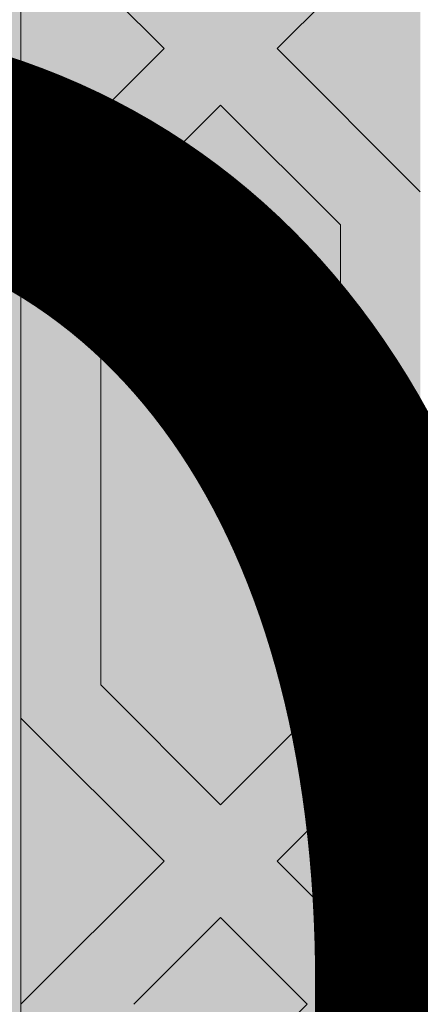
# Model space of a CAD drawing. Units: inches. Extents: x 844 to 2234, y 346 to 1084.
# Tile 75 of 93: x 1997.478 to 1998.757, y 701.365 to 704.51. Entities that reach past the tile are written whole.
import ezdxf

# ---------------------------------------------------------------- set-up
doc = ezdxf.new("R2010")
doc.units = ezdxf.units.IN
doc.header["$MEASUREMENT"] = 0
for name, color, linetype, lineweight in [('A-ANNO-DIMS', 2, 'Continuous', 18), ('furniture', 8, 'Continuous', 18), ('RA-AP-01$0$INT', 35, 'Continuous', 5)]:
    doc.layers.add(name, color=color, linetype=linetype, lineweight=lineweight)
doc.layers.add('RA-AP-01$0$FURN', color=3, linetype='Continuous')
doc.styles.get("Standard").update_dxf_attribs({"font": 'arial.ttf'})
doc.dimstyles.get("Standard").update_dxf_attribs({"dimtxt": 6, "dimasz": 3, "dimexe": 0.18, "dimexo": 0.0625, "dimgap": 0.09, "dimtad": 0, "dimtih": 1, "dimtoh": 1, "dimdec": 1, "dimzin": 0, "dimdsep": 46, "dimlunit": 3, "dimtxsty": 'Standard', "dimblk": 'ARCHTICK', "dimcen": 0.09, "dimadec": 0, "dimazin": 0, "dimtfac": 1, "dimtdec": 1, "dimtofl": 0, "dimtmove": 0, "dimatfit": 3, "dimfxl": 1, "dimtolj": 1, "dimtzin": 0, "dimarcsym": 0})

# ---------------------------------------------------------------- blocks, each defined once
blk = doc.blocks.new('A$C18D01794')
at = {"layer": 'RA-AP-01$0$INT'}
h = blk.add_hatch(color=256, dxfattribs=at)
h.paths.add_polyline_path([(4.35521, -6.15671), (4.35521, -8.05671), (5.45521, -8.05671), (5.45521, -6.15671)])
h.paths.add_polyline_path([(4.40521, -8.00671), (4.40521, -6.20671), (5.40521, -6.20671), (5.40521, -8.00671)], flags=16)
h = blk.add_hatch(color=256, dxfattribs=at)
h.paths.add_polyline_path([(4.46935, -7.07085), (4.50521, -7.035), (4.50521, -7.10671)])
h.paths.add_polyline_path([(4.45521, -7.085), (4.47692, -7.10671), (4.43349, -7.10671)])
h.paths.add_polyline_path([(4.40521, -7.035), (4.44106, -7.07085), (4.40521, -7.10671)])
h.paths.add_polyline_path([(4.42521, -6.91146), (4.45521, -6.88146), (4.48521, -6.91146), (4.48521, -7.02671), (4.45521, -7.05671), (4.42521, -7.02671)])
h.paths.add_polyline_path([(4.50521, -6.83146), (4.50521, -6.90318), (4.46935, -6.86732)])
h.paths.add_polyline_path([(4.42521, -6.70793), (4.45521, -6.67793), (4.48521, -6.70793), (4.48521, -6.82318), (4.45521, -6.85318), (4.42521, -6.82318)])
h.paths.add_polyline_path([(4.42521, -6.50439), (4.45521, -6.47439), (4.48521, -6.50439), (4.48521, -6.61964), (4.45521, -6.64964), (4.42521, -6.61964)])
h.paths.add_polyline_path([(4.46935, -6.66378), (4.50521, -6.62793), (4.50521, -6.69964)])
h.paths.add_polyline_path([(4.40521, -6.62793), (4.44106, -6.66378), (4.40521, -6.69964)])
h.paths.add_polyline_path([(4.40521, -6.42439), (4.44106, -6.46025), (4.40521, -6.49611)])
h.paths.add_polyline_path([(4.46935, -6.46025), (4.50521, -6.42439), (4.50521, -6.49611)])
h.paths.add_polyline_path([(4.42521, -6.30085), (4.45521, -6.27085), (4.48521, -6.30085), (4.48521, -6.41611), (4.45521, -6.44611), (4.42521, -6.41611)])
h.paths.add_polyline_path([(4.42521, -6.22671), (4.47106, -6.22671), (4.42521, -6.27257)])
h.paths.add_polyline_path([(4.49935, -6.22671), (4.63606, -6.22671), (4.66606, -6.25671), (4.63606, -6.28671), (4.49935, -6.28671), (4.46935, -6.25671)])
h.paths.add_polyline_path([(4.68021, -6.27085), (4.71606, -6.30671), (4.64435, -6.30671)])
h.paths.add_polyline_path([(4.64435, -6.20671), (4.71606, -6.20671), (4.68021, -6.24257)])
h.paths.add_polyline_path([(4.72435, -6.22671), (4.86106, -6.22671), (4.89106, -6.25671), (4.86106, -6.28671), (4.72435, -6.28671), (4.69435, -6.25671)])
h.paths.add_polyline_path([(4.90521, -6.27085), (4.94106, -6.30671), (4.86935, -6.30671)])
h.paths.add_polyline_path([(4.86935, -6.20671), (4.94106, -6.20671), (4.90521, -6.24257)])
h.paths.add_polyline_path([(4.94935, -6.22671), (5.08606, -6.22671), (5.11606, -6.25671), (5.08606, -6.28671), (4.94935, -6.28671), (4.91935, -6.25671)])
h.paths.add_polyline_path([(5.13021, -6.27085), (5.16606, -6.30671), (5.09435, -6.30671)])
h.paths.add_polyline_path([(5.09435, -6.20671), (5.16606, -6.20671), (5.13021, -6.24257)])
h.paths.add_polyline_path([(5.17435, -6.22671), (5.31106, -6.22671), (5.34106, -6.25671), (5.31106, -6.28671), (5.17435, -6.28671), (5.14435, -6.25671)])
h.paths.add_polyline_path([(5.32521, -6.30085), (5.35521, -6.27085), (5.38521, -6.30085), (5.38521, -6.41611), (5.35521, -6.44611), (5.32521, -6.41611)])
h.paths.add_polyline_path([(5.33935, -6.22671), (5.38521, -6.22671), (5.38521, -6.27257)])
h.paths.add_polyline_path([(5.32521, -6.50439), (5.35521, -6.47439), (5.38521, -6.50439), (5.38521, -6.61964), (5.35521, -6.64964), (5.32521, -6.61964)])
h.paths.add_polyline_path([(5.30521, -6.42439), (5.34106, -6.46025), (5.30521, -6.49611)])
h.paths.add_polyline_path([(5.36935, -6.46025), (5.40521, -6.42439), (5.40521, -6.49611)])
h.paths.add_polyline_path([(5.40521, -6.62793), (5.40521, -6.69964), (5.36935, -6.66378)])
h.paths.add_polyline_path([(5.30521, -6.62793), (5.34106, -6.66378), (5.30521, -6.69964)])
h.paths.add_polyline_path([(5.32521, -6.70793), (5.35521, -6.67793), (5.38521, -6.70793), (5.38521, -6.82318), (5.35521, -6.85318), (5.32521, -6.82318)])
h.paths.add_polyline_path([(5.30521, -6.83146), (5.34106, -6.86732), (5.30521, -6.90318)])
h.paths.add_polyline_path([(5.32521, -6.91146), (5.35521, -6.88146), (5.38521, -6.91146), (5.38521, -7.02671), (5.35521, -7.05671), (5.32521, -7.02671)])
h.paths.add_polyline_path([(5.40458, -6.83209, 0.001218), (5.40521, -6.83231), (5.40521, -6.90318), (5.36935, -6.86732)])
h.paths.add_polyline_path([(5.36935, -7.07085), (5.40521, -7.035), (5.40521, -7.10671)])
h.paths.add_polyline_path([(5.35521, -7.085), (5.37692, -7.10671), (5.33349, -7.10671)])
h.paths.add_polyline_path([(5.30521, -7.035), (5.34106, -7.07085), (5.30521, -7.10671)])
h = blk.add_hatch(color=256, dxfattribs=at)
h.paths.add_polyline_path([(4.50521, -6.62793), (4.46935, -6.66378), (4.50521, -6.69964), (4.50521, -6.83146), (4.46935, -6.86732), (4.50521, -6.90318), (4.50521, -7.035), (4.46935, -7.07085), (4.50521, -7.10671), (4.47692, -7.10671), (4.45521, -7.085), (4.43349, -7.10671), (4.40521, -7.10671), (4.44106, -7.07085), (4.40521, -7.035), (4.40521, -6.90318), (4.44106, -6.86732), (4.40521, -6.83146), (4.40521, -6.69964), (4.44106, -6.66378), (4.40521, -6.62793), (4.40521, -6.49611), (4.44106, -6.46025), (4.40521, -6.42439), (4.40521, -6.20671), (4.64435, -6.20671), (4.68021, -6.24257), (4.71606, -6.20671), (4.86935, -6.20671), (4.90521, -6.24257), (4.94106, -6.20671), (5.09435, -6.20671), (5.13021, -6.24257), (5.16606, -6.20671), (5.40521, -6.20671), (5.40521, -6.42439), (5.36935, -6.46025), (5.40521, -6.49611), (5.40521, -6.62793), (5.36935, -6.66378), (5.40521, -6.69964), (5.40521, -6.83146), (5.36935, -6.86732), (5.40521, -6.90318), (5.40521, -7.035), (5.36935, -7.07085), (5.40521, -7.10671), (5.37692, -7.10671), (5.35521, -7.085), (5.33349, -7.10671), (5.30521, -7.10671), (5.34106, -7.07085), (5.30521, -7.035), (5.30521, -6.90318), (5.34106, -6.86732), (5.30521, -6.83146), (5.30521, -6.69964), (5.34106, -6.66378), (5.30521, -6.62793), (5.30521, -6.49611), (5.34106, -6.46025), (5.30521, -6.42439), (5.30521, -6.30671), (5.16606, -6.30671), (5.13021, -6.27085), (5.09435, -6.30671), (4.94106, -6.30671), (4.90521, -6.27085), (4.86935, -6.30671), (4.71606, -6.30671), (4.68021, -6.27085), (4.64435, -6.30671), (4.50521, -6.30671), (4.50521, -6.42439), (4.46935, -6.46025), (4.50521, -6.49611)])
h.paths.add_polyline_path([(4.48521, -6.50439), (4.45521, -6.47439), (4.42521, -6.50439), (4.42521, -6.61964), (4.45521, -6.64964), (4.48521, -6.61964)], flags=16)
h.paths.add_polyline_path([(4.45521, -6.44611), (4.48521, -6.41611), (4.48521, -6.30085), (4.45521, -6.27085), (4.42521, -6.30085), (4.42521, -6.41611)], flags=16)
h.paths.add_polyline_path([(4.45521, -6.67793), (4.42521, -6.70793), (4.42521, -6.82318), (4.45521, -6.85318), (4.48521, -6.82318), (4.48521, -6.70793)], flags=16)
h.paths.add_polyline_path([(4.49935, -6.28671), (4.63606, -6.28671), (4.66606, -6.25671), (4.63606, -6.22671), (4.49935, -6.22671), (4.46935, -6.25671)], flags=16)
h.paths.add_polyline_path([(4.42521, -6.27257), (4.47106, -6.22671), (4.42521, -6.22671)], flags=16)
h.paths.add_polyline_path([(4.45521, -6.88146), (4.42521, -6.91146), (4.42521, -7.02671), (4.45521, -7.05671), (4.48521, -7.02671), (4.48521, -6.91146)], flags=16)
h.paths.add_polyline_path([(4.72435, -6.28671), (4.86106, -6.28671), (4.89106, -6.25671), (4.86106, -6.22671), (4.72435, -6.22671), (4.69435, -6.25671)], flags=16)
h.paths.add_polyline_path([(4.91935, -6.25671), (4.94935, -6.28671), (5.08606, -6.28671), (5.11606, -6.25671), (5.08606, -6.22671), (4.94935, -6.22671)], flags=16)
h.paths.add_polyline_path([(5.14435, -6.25671), (5.17435, -6.28671), (5.31106, -6.28671), (5.34106, -6.25671), (5.31106, -6.22671), (5.17435, -6.22671)], flags=16)
h.paths.add_polyline_path([(5.32521, -6.61964), (5.35521, -6.64964), (5.38521, -6.61964), (5.38521, -6.50439), (5.35521, -6.47439), (5.32521, -6.50439)], flags=16)
h.paths.add_polyline_path([(5.32521, -6.41611), (5.35521, -6.44611), (5.38521, -6.41611), (5.38521, -6.30085), (5.35521, -6.27085), (5.32521, -6.30085)], flags=16)
h.paths.add_polyline_path([(5.32521, -6.70793), (5.32521, -6.82318), (5.35521, -6.85318), (5.38521, -6.82318), (5.38521, -6.70793), (5.35521, -6.67793)], flags=16)
h.paths.add_polyline_path([(5.32521, -6.91146), (5.32521, -7.02671), (5.35521, -7.05671), (5.38521, -7.02671), (5.38521, -6.91146), (5.35521, -6.88146)], flags=16)
h.paths.add_polyline_path([(5.33935, -6.22671), (5.38521, -6.27257), (5.38521, -6.22671)], flags=16)
h = blk.add_hatch(color=256, dxfattribs=at)
h.paths.add_polyline_path([(4.50521, -7.5855), (4.46935, -7.54964), (4.50521, -7.51378), (4.50521, -7.38196), (4.46935, -7.34611), (4.50521, -7.31025), (4.50521, -7.17843), (4.46935, -7.14257), (4.50521, -7.10671), (4.47692, -7.10671), (4.45521, -7.12843), (4.43349, -7.10671), (4.40521, -7.10671), (4.44106, -7.14257), (4.40521, -7.17843), (4.40521, -7.31025), (4.44106, -7.34611), (4.40521, -7.38196), (4.40521, -7.51378), (4.44106, -7.54964), (4.40521, -7.5855), (4.40521, -7.71732), (4.44106, -7.75318), (4.40521, -7.78903), (4.40521, -8.00671), (4.64435, -8.00671), (4.68021, -7.97085), (4.71606, -8.00671), (4.86935, -8.00671), (4.90521, -7.97085), (4.94106, -8.00671), (5.09435, -8.00671), (5.13021, -7.97085), (5.16606, -8.00671), (5.40521, -8.00671), (5.40521, -7.78903), (5.36935, -7.75318), (5.40521, -7.71732), (5.40521, -7.5855), (5.36935, -7.54964), (5.40521, -7.51378), (5.40521, -7.38196), (5.36935, -7.34611), (5.40521, -7.31025), (5.40521, -7.17843), (5.36935, -7.14257), (5.40521, -7.10671), (5.37692, -7.10671), (5.35521, -7.12843), (5.33349, -7.10671), (5.30521, -7.10671), (5.34106, -7.14257), (5.30521, -7.17843), (5.30521, -7.31025), (5.34106, -7.34611), (5.30521, -7.38196), (5.30521, -7.51378), (5.34106, -7.54964), (5.30521, -7.5855), (5.30521, -7.71732), (5.34106, -7.75318), (5.30521, -7.78903), (5.30521, -7.90671), (5.16606, -7.90671), (5.13021, -7.94257), (5.09435, -7.90671), (4.94106, -7.90671), (4.90521, -7.94257), (4.86935, -7.90671), (4.71606, -7.90671), (4.68021, -7.94257), (4.64435, -7.90671), (4.50521, -7.90671), (4.50521, -7.78903), (4.46935, -7.75318), (4.50521, -7.71732)])
h.paths.add_polyline_path([(4.48521, -7.70903), (4.45521, -7.73903), (4.42521, -7.70903), (4.42521, -7.59378), (4.45521, -7.56378), (4.48521, -7.59378)], flags=16)
h.paths.add_polyline_path([(4.45521, -7.76732), (4.48521, -7.79732), (4.48521, -7.91257), (4.45521, -7.94257), (4.42521, -7.91257), (4.42521, -7.79732)], flags=16)
h.paths.add_polyline_path([(4.45521, -7.5355), (4.42521, -7.5055), (4.42521, -7.39025), (4.45521, -7.36025), (4.48521, -7.39025), (4.48521, -7.5055)], flags=16)
h.paths.add_polyline_path([(4.49935, -7.92671), (4.63606, -7.92671), (4.66606, -7.95671), (4.63606, -7.98671), (4.49935, -7.98671), (4.46935, -7.95671)], flags=16)
h.paths.add_polyline_path([(4.42521, -7.94085), (4.47106, -7.98671), (4.42521, -7.98671)], flags=16)
h.paths.add_polyline_path([(4.45521, -7.33196), (4.42521, -7.30196), (4.42521, -7.18671), (4.45521, -7.15671), (4.48521, -7.18671), (4.48521, -7.30196)], flags=16)
h.paths.add_polyline_path([(4.72435, -7.92671), (4.86106, -7.92671), (4.89106, -7.95671), (4.86106, -7.98671), (4.72435, -7.98671), (4.69435, -7.95671)], flags=16)
h.paths.add_polyline_path([(4.91935, -7.95671), (4.94935, -7.92671), (5.08606, -7.92671), (5.11606, -7.95671), (5.08606, -7.98671), (4.94935, -7.98671)], flags=16)
h.paths.add_polyline_path([(5.14435, -7.95671), (5.17435, -7.92671), (5.31106, -7.92671), (5.34106, -7.95671), (5.31106, -7.98671), (5.17435, -7.98671)], flags=16)
h.paths.add_polyline_path([(5.32521, -7.59378), (5.35521, -7.56378), (5.38521, -7.59378), (5.38521, -7.70903), (5.35521, -7.73903), (5.32521, -7.70903)], flags=16)
h.paths.add_polyline_path([(5.32521, -7.79732), (5.35521, -7.76732), (5.38521, -7.79732), (5.38521, -7.91257), (5.35521, -7.94257), (5.32521, -7.91257)], flags=16)
h.paths.add_polyline_path([(5.32521, -7.5055), (5.32521, -7.39025), (5.35521, -7.36025), (5.38521, -7.39025), (5.38521, -7.5055), (5.35521, -7.5355)], flags=16)
h.paths.add_polyline_path([(5.32521, -7.30196), (5.32521, -7.18671), (5.35521, -7.15671), (5.38521, -7.18671), (5.38521, -7.30196), (5.35521, -7.33196)], flags=16)
h.paths.add_polyline_path([(5.33935, -7.98671), (5.38521, -7.94085), (5.38521, -7.98671)], flags=16)
h = blk.add_hatch(color=256, dxfattribs=at)
h.paths.add_polyline_path([(4.46935, -7.14257), (4.50521, -7.17843), (4.50521, -7.10671)])
h.paths.add_polyline_path([(4.45521, -7.12843), (4.47692, -7.10671), (4.43349, -7.10671)])
h.paths.add_polyline_path([(4.40521, -7.17843), (4.44106, -7.14257), (4.40521, -7.10671)])
h.paths.add_polyline_path([(4.42521, -7.30196), (4.45521, -7.33196), (4.48521, -7.30196), (4.48521, -7.18671), (4.45521, -7.15671), (4.42521, -7.18671)])
h.paths.add_polyline_path([(4.50521, -7.38196), (4.50521, -7.31025), (4.46935, -7.34611)])
h.paths.add_polyline_path([(4.42521, -7.5055), (4.45521, -7.5355), (4.48521, -7.5055), (4.48521, -7.39025), (4.45521, -7.36025), (4.42521, -7.39025)])
h.paths.add_polyline_path([(4.42521, -7.70903), (4.45521, -7.73903), (4.48521, -7.70903), (4.48521, -7.59378), (4.45521, -7.56378), (4.42521, -7.59378)])
h.paths.add_polyline_path([(4.46935, -7.54964), (4.50521, -7.5855), (4.50521, -7.51378)])
h.paths.add_polyline_path([(4.40521, -7.5855), (4.44106, -7.54964), (4.40521, -7.51378)])
h.paths.add_polyline_path([(4.40521, -7.78903), (4.44106, -7.75318), (4.40521, -7.71732)])
h.paths.add_polyline_path([(4.46935, -7.75318), (4.50521, -7.78903), (4.50521, -7.71732)])
h.paths.add_polyline_path([(4.42521, -7.91257), (4.45521, -7.94257), (4.48521, -7.91257), (4.48521, -7.79732), (4.45521, -7.76732), (4.42521, -7.79732)])
h.paths.add_polyline_path([(4.42521, -7.98671), (4.47106, -7.98671), (4.42521, -7.94085)])
h.paths.add_polyline_path([(4.49935, -7.98671), (4.63606, -7.98671), (4.66606, -7.95671), (4.63606, -7.92671), (4.49935, -7.92671), (4.46935, -7.95671)])
h.paths.add_polyline_path([(4.68021, -7.94257), (4.71606, -7.90671), (4.64435, -7.90671)])
h.paths.add_polyline_path([(4.64435, -8.00671), (4.71606, -8.00671), (4.68021, -7.97085)])
h.paths.add_polyline_path([(4.72435, -7.98671), (4.86106, -7.98671), (4.89106, -7.95671), (4.86106, -7.92671), (4.72435, -7.92671), (4.69435, -7.95671)])
h.paths.add_polyline_path([(4.90521, -7.94257), (4.94106, -7.90671), (4.86935, -7.90671)])
h.paths.add_polyline_path([(4.86935, -8.00671), (4.94106, -8.00671), (4.90521, -7.97085)])
h.paths.add_polyline_path([(4.94935, -7.98671), (5.08606, -7.98671), (5.11606, -7.95671), (5.08606, -7.92671), (4.94935, -7.92671), (4.91935, -7.95671)])
h.paths.add_polyline_path([(5.13021, -7.94257), (5.16606, -7.90671), (5.09435, -7.90671)])
h.paths.add_polyline_path([(5.09435, -8.00671), (5.16606, -8.00671), (5.13021, -7.97085)])
h.paths.add_polyline_path([(5.17435, -7.98671), (5.31106, -7.98671), (5.34106, -7.95671), (5.31106, -7.92671), (5.17435, -7.92671), (5.14435, -7.95671)])
h.paths.add_polyline_path([(5.32521, -7.91257), (5.35521, -7.94257), (5.38521, -7.91257), (5.38521, -7.79732), (5.35521, -7.76732), (5.32521, -7.79732)])
h.paths.add_polyline_path([(5.33935, -7.98671), (5.38521, -7.98671), (5.38521, -7.94085)])
h.paths.add_polyline_path([(5.32521, -7.70903), (5.35521, -7.73903), (5.38521, -7.70903), (5.38521, -7.59378), (5.35521, -7.56378), (5.32521, -7.59378)])
h.paths.add_polyline_path([(5.30521, -7.78903), (5.34106, -7.75318), (5.30521, -7.71732)])
h.paths.add_polyline_path([(5.36935, -7.75318), (5.40521, -7.78903), (5.40521, -7.71732)])
h.paths.add_polyline_path([(5.40521, -7.5855), (5.40521, -7.51378), (5.36935, -7.54964)])
h.paths.add_polyline_path([(5.30521, -7.5855), (5.34106, -7.54964), (5.30521, -7.51378)])
h.paths.add_polyline_path([(5.32521, -7.5055), (5.35521, -7.5355), (5.38521, -7.5055), (5.38521, -7.39025), (5.35521, -7.36025), (5.32521, -7.39025)])
h.paths.add_polyline_path([(5.30521, -7.38196), (5.34106, -7.34611), (5.30521, -7.31025)])
h.paths.add_polyline_path([(5.32521, -7.30196), (5.35521, -7.33196), (5.38521, -7.30196), (5.38521, -7.18671), (5.35521, -7.15671), (5.32521, -7.18671)])
h.paths.add_polyline_path([(5.40458, -7.38134, -0.001218), (5.40521, -7.38111), (5.40521, -7.31025), (5.36935, -7.34611)])
h.paths.add_polyline_path([(5.36935, -7.14257), (5.40521, -7.17843), (5.40521, -7.10671)])
h.paths.add_polyline_path([(5.35521, -7.12843), (5.37692, -7.10671), (5.33349, -7.10671)])
h.paths.add_polyline_path([(5.30521, -7.17843), (5.34106, -7.14257), (5.30521, -7.10671)])
for p, q in [((5.34106, -7.07085), (5.30521, -7.10671)), ((5.35521, -7.085), (5.33349, -7.10671)), ((5.34106, -7.14257), (5.30521, -7.10671)), ((5.35521, -7.12843), (5.33349, -7.10671)), ((5.35521, -7.12843), (5.37692, -7.10671)), ((5.36935, -7.14257), (5.40521, -7.10671)), ((5.30521, -7.17843), (5.34106, -7.14257)), ((5.40521, -7.17843), (5.36935, -7.14257)), ((5.32521, -7.18671), (5.35521, -7.15671)), ((5.38521, -7.18671), (5.35521, -7.15671)), ((5.32521, -7.30196), (5.32521, -7.18671)), ((5.38521, -7.30196), (5.38521, -7.18671)), ((5.32521, -7.30196), (5.35521, -7.33196)), ((5.38521, -7.30196), (5.35521, -7.33196)), ((5.30521, -7.31025), (5.34106, -7.34611)), ((5.40521, -7.31025), (5.36935, -7.34611)), ((5.30521, -7.38196), (5.34106, -7.34611)), ((5.40521, -7.38196), (5.36935, -7.34611))]:
    blk.add_line(p, q, dxfattribs=at)
for points in [[(5.40521, -7.10671), (5.40521, -6.20671)], [(5.40521, -7.10671), (5.40521, -8.00671)]]:
    blk.add_lwpolyline(points, dxfattribs=at)
blk = doc.blocks.new('A$C5D2F253E')
at = {"layer": 'RA-AP-01$0$FURN', "xscale": -0.7999999999883585, "yscale": 0.7999999999883585, "zscale": 0.8, "rotation": 90}
blk.add_blockref('A$C18D01794', (-5.68776, 4.75792), dxfattribs=at)
blk = doc.blocks.new('_ArchTick')
at = {"color": 0, "linetype": 'ByBlock', "const_width": 0.15}
blk.add_lwpolyline([(-0.5, -0.5), (0.5, 0.5)], dxfattribs=at)
blk = doc.blocks.new('*D121')
at = {"layer": 'A-ANNO-DIMS', "color": 0, "lineweight": -2, "transparency": 16777216}
for p, q in [((2030.272, 734.2626), (2040.2453, 734.2626)), ((2040.0653, 734.2626), (2040.0653, 704.6044)), ((2040.0653, 668.5574), (2040.0653, 698.2156)), ((2030.272, 668.5574), (2040.2453, 668.5574))]:
    blk.add_line(p, q, dxfattribs=at)
at = {"layer": 'Defpoints', "color": 0, "transparency": 16777216}
for p in [(2030.2095, 734.2626), (2040.0653, 734.2626), (2030.2095, 668.5574)]:
    blk.add_point(p, dxfattribs=at)
at = {"layer": 'A-ANNO-DIMS', "color": 0, "lineweight": -2, "transparency": 16777216, "xscale": 3, "yscale": 3, "zscale": 3}
for p, rotation in [((2040.0653, 734.2626), 90), ((2040.0653, 668.5574), 270)]:
    blk.add_blockref('_ArchTick', p, dxfattribs=dict(at, rotation=rotation))
at = {"layer": 'A-ANNO-DIMS', "color": 0, "transparency": 16777216, "insert": (2040.0653, 701.41), "char_height": 6, "attachment_point": 5}
blk.add_mtext('\\A1;LOUNGE SET 5\'-5 1/2" TYP.', dxfattribs=at)

msp = doc.modelspace()

# ---------------------------------------------------------------- block references
at = {"layer": 'furniture', "xscale": -15.94108302203742, "yscale": 15.94108302203742, "zscale": 15.94108302203742, "rotation": 270}
msp.add_blockref('A$C5D2F253E', (1990.5673, 701.4029), dxfattribs=at)

# ---------------------------------------------------------------- dimensions: what is measured, and where the dimension line sits
at = {"layer": 'A-ANNO-DIMS'}
dim = msp.add_linear_dim(base=(2040.0653, 734.2626), p1=(2030.2095, 668.5574), p2=(2030.2095, 734.2626), angle=90, text='LOUNGE SET <> TYP.', dimstyle='Standard', override={"dimdec": 1, "dimlfac": 1, "dimrnd": 0, "dimzin": 1, "dimdsep": 46, "dimlunit": 4, "dimfrac": 2}, dxfattribs=at)
dim.commit()
dim.dimension.update_dxf_attribs({"geometry": '*D121', "text_midpoint": (2040.0653, 701.41)})

doc.saveas('drawing.dxf')
